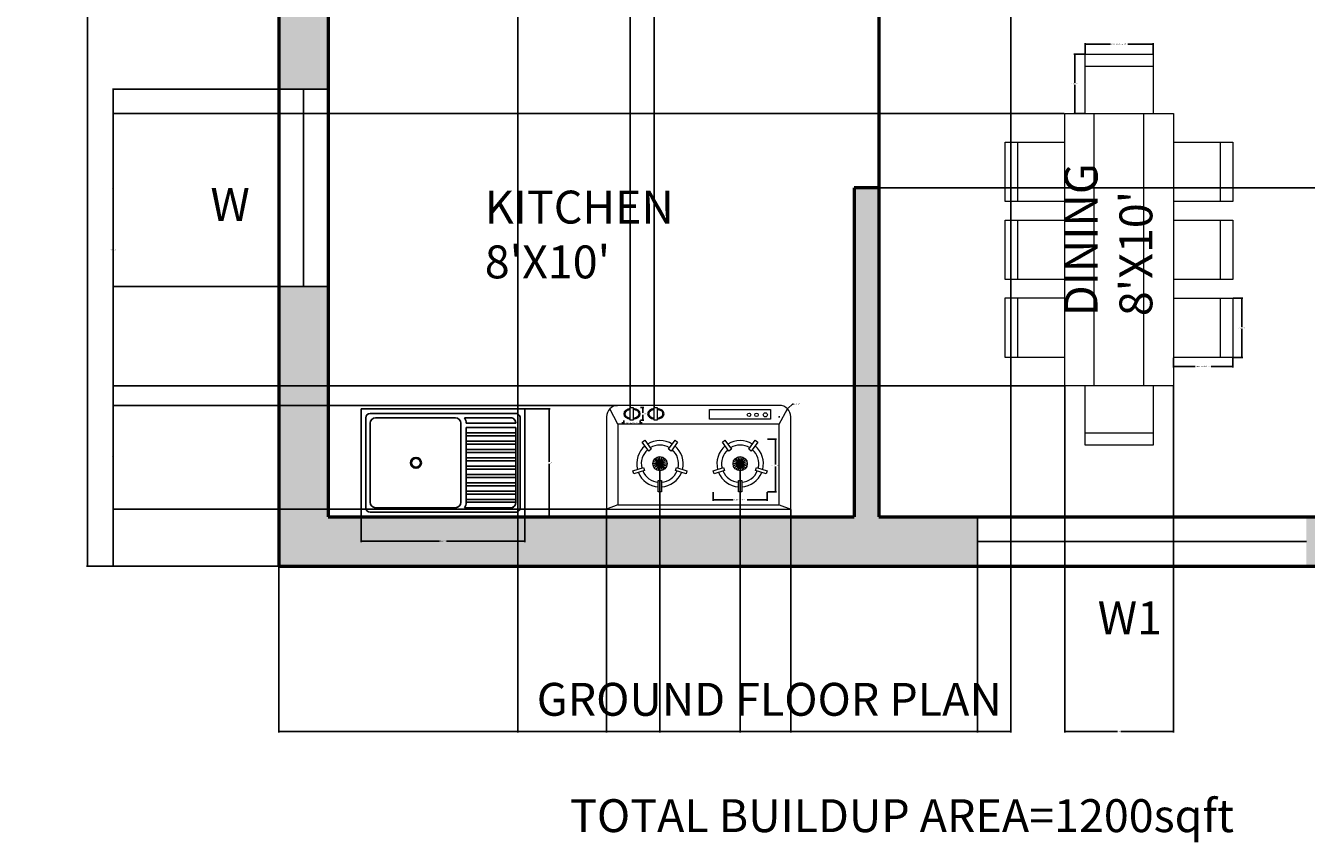
# Model space of a CAD drawing. Units: inches. Extents: x -15 to 420, y -514 to 86.
# Tile 1 of 8: x -15 to 218, y -514 to -365. Entities that reach past the tile are written whole.
import ezdxf

# ---------------------------------------------------------------- set-up
doc = ezdxf.new("R2010")
doc.units = ezdxf.units.IN
doc.header["$MEASUREMENT"] = 0
for name, color, linetype, lineweight in [('A-ANNO-DIMS', 2, 'Continuous', 18), ('A-ANNO-TEXT', 7, 'Continuous', 18), ('A-AREA-IDEN', 7, 'Continuous', 25), ('A-EQPM', 8, 'Continuous', 18), ('A-FLOR-FIXT', 9, 'Continuous', 25), ('A-FURN', 8, 'Continuous', 18), ('A-GLAZ', 41, 'Continuous', 25), ('A-WALL', 7, 'Continuous', 50), ('A-WALL-PATT', 8, 'Continuous', 13)]:
    doc.layers.add(name, color=color, linetype=linetype, lineweight=lineweight)
doc.styles.get("Standard").update_dxf_attribs({"font": 'arial.ttf'})
doc.dimstyles.get("Standard").update_dxf_attribs({"dimtxt": 0.18, "dimasz": 0.18, "dimexe": 0.18, "dimexo": 0.0625, "dimgap": 0.09, "dimtad": 0, "dimtih": 1, "dimtoh": 1, "dimdec": 0, "dimzin": 0, "dimdsep": 46, "dimlunit": 3, "dimtxsty": 'Standard', "dimcen": 0.09, "dimadec": 0, "dimazin": 0, "dimtfac": 1, "dimtdec": 0, "dimtofl": 0, "dimtmove": 0, "dimatfit": 3, "dimfxl": 1, "dimtolj": 1, "dimtzin": 0, "dimarcsym": 0})

# ---------------------------------------------------------------- blocks, each defined once
blk = doc.blocks.new('*D2')
at = {"layer": 'A-ANNO-DIMS', "color": 0, "lineweight": -2, "transparency": 16777216}
for p, q in [((30.86, 13.12), (-4.15, 13.12)), ((-3.97, 12.94), (-3.97, -222.22)), ((-3.97, -463.7), (-3.97, -228.53)), ((30.86, -463.88), (-4.15, -463.88))]:
    blk.add_line(p, q, dxfattribs=at)
at = {"layer": 'A-ANNO-DIMS', "color": 0, "transparency": 16777216}
for points in [[(-4, 12.94), (-3.94, 12.94), (-3.97, 13.12)], [(-4, -463.7), (-3.94, -463.7), (-3.97, -463.88)]]:
    blk.add_solid(points, dxfattribs=at)
at = {"layer": 'Defpoints', "color": 0, "transparency": 16777216}
for p in [(30.92, 13.12), (-3.97, -463.88), (30.92, -463.88)]:
    blk.add_point(p, dxfattribs=at)
at = {"layer": 'A-ANNO-DIMS', "color": 0, "transparency": 16777216, "insert": (-3.97, -225.38), "char_height": 6, "attachment_point": 5}
blk.add_mtext('\\A1;39\'-9"', dxfattribs=at)
blk = doc.blocks.new('М12 540х820')
for p, q in [((0, 540), (-820, 540)), ((-820, 540), (-820, 0)), ((-45, 517.5), (-775, 517.5)), ((0, 0), (0, 540)), ((-797.5, 495), (-797.5, 45)), ((-775, 468), (-775, 72)), ((-347.5, 495), (-748, 495)), ((-320.5, 468), (-320.5, 72)), ((-301.7, 495), (-64.8, 495)), ((-293.7, 468), (-293.7, 472.5)), ((-293.7, 468), (-45, 468)), ((-45, 469.5), (-45, 468)), ((-22.5, 45), (-22.5, 495)), ((-293.7, 446.6), (-45, 446.6)), ((-293.7, 419.6), (-293.7, 446.6)), ((-293.7, 419.6), (-45, 419.6)), ((-293.7, 405), (-45, 405)), ((-293.7, 378), (-293.7, 405)), ((-45, 419.6), (-45, 446.6)), ((-45, 378), (-45, 405)), ((-293.7, 378), (-45, 378)), ((-293.7, 336.4), (-293.7, 363.4)), ((-293.7, 363.4), (-45, 363.4)), ((-293.7, 336.4), (-45, 336.4)), ((-293.7, 294.7), (-293.7, 321.7)), ((-293.7, 321.7), (-45, 321.7)), ((-45, 336.4), (-45, 363.4)), ((-45, 294.7), (-45, 321.7)), ((-293.7, 294.7), (-45, 294.7)), ((-293.7, 253.1), (-293.7, 280.1)), ((-293.7, 280.1), (-45, 280.1)), ((-45, 253.1), (-45, 280.1)), ((-293.7, 253.1), (-45, 253.1)), ((-293.7, 211.5), (-293.7, 238.5)), ((-293.7, 238.5), (-45, 238.5)), ((-293.7, 211.5), (-45, 211.5)), ((-293.7, 169.9), (-293.7, 196.9)), ((-293.7, 196.9), (-45, 196.9)), ((-45, 211.5), (-45, 238.5)), ((-45, 169.9), (-45, 196.9)), ((-293.7, 169.9), (-45, 169.9)), ((-293.7, 128.2), (-293.7, 155.2)), ((-293.7, 155.2), (-45, 155.2)), ((-45, 128.2), (-45, 155.2)), ((-293.7, 128.2), (-45, 128.2)), ((-293.7, 113.6), (-45, 113.6)), ((-293.7, 86.6), (-293.7, 113.6)), ((-293.7, 86.6), (-45, 86.6)), ((-293.7, 72), (-45, 72)), ((-45, 86.6), (-45, 113.6)), ((-45, 70.5), (-45, 72)), ((-820, 0), (0, 0)), ((-775, 22.5), (-45, 22.5)), ((-748, 45), (-347.5, 45)), ((-301.7, 45), (-64.8, 45))]:
    blk.add_line(p, q)
at = {"ltscale": 0.06}
for p, q in [((-820, 0), (-820, 540)), ((-820, 540), (0, 540)), ((0, 540), (0, 536.9)), ((0, 536.9), (0, 0)), ((-293.7, 446.6), (-45, 446.6)), ((-293.7, 405), (-293.7, 446.6)), ((-293.7, 363.4), (-293.7, 405)), ((-45, 446.6), (-45, 419.6)), ((-45, 419.6), (-45, 378)), ((-293.7, 321.7), (-293.7, 363.4)), ((-293.7, 280.1), (-293.7, 321.7)), ((-45, 378), (-45, 336.4)), ((-45, 336.4), (-45, 294.7)), ((-293.7, 238.5), (-293.7, 280.1)), ((-45, 294.7), (-45, 253.1)), ((-293.7, 196.9), (-293.7, 238.5)), ((-293.7, 155.2), (-293.7, 196.9)), ((-45, 253.1), (-45, 211.5)), ((-45, 211.5), (-45, 169.9)), ((-293.7, 113.6), (-293.7, 155.2)), ((-45, 169.9), (-45, 128.2)), ((-293.7, 72), (-293.7, 113.6)), ((-45, 72), (-293.7, 72)), ((-45, 128.2), (-45, 86.6)), ((-45, 86.6), (-45, 72)), ((0, 0), (-820, 0))]:
    blk.add_line(p, q, dxfattribs=at)
at = {"extrusion": (0, 0, -1)}
for centre, major_axis, start_param, end_param in [((-775, 495), (-15.9, 15.9), -0.785398, 0.785398), ((-775, 495), (-15.9, 15.9), -0.785398, 0.785398), ((-45, 495), (-15.9, -15.9), 2.356194, 3.926991), ((-45, 495), (-15.9, -15.9), 2.356194, 3.926991), ((-748, 468), (-19.1, -19.1), 0.785398, 2.356194), ((-748, 468), (-19.1, -19.1), 0.785398, 2.356194), ((-347.5, 468), (-19.1, 19.1), 0.785398, 2.356194), ((-347.5, 468), (-19.1, 19.1), 0.785398, 2.356194), ((-343.2, 468), (-35, 35), 1.779263, 2.356194), ((-343.2, 468), (-35, 35), 1.779263, 2.356192), ((-343.2, 468), (-35, 35), 2.356192, 2.356194), ((-72.3, 468.8), (-19.3, 19.3), 1.0328, 2.38382), ((-72.3, 468.8), (-19.3, 19.3), 1.0328, 1.064673), ((-72.3, 468.8), (-19.3, 19.3), 1.064673, 2.328569), ((-72.3, 468.8), (-19.3, 19.3), 2.328569, 2.38382), ((-545.5, 270), (-19.1, -19.1), 3.926991, 10.210176), ((-545.5, 270), (-19.1, -19.1), 3.926991, 10.210176), ((-545.5, 270), (-15.9, -15.9), 3.926991, 10.210176), ((-545.5, 270), (-15.9, -15.9), 3.926991, 10.210176), ((-748, 72), (-19.1, 19.1), 3.926991, 5.497787), ((-748, 72), (-19.1, 19.1), 3.926991, 5.497787), ((-347.5, 72), (-19.1, -19.1), 3.926991, 5.497787), ((-347.5, 72), (-19.1, -19.1), 3.926991, 5.497787), ((-343.2, 72), (-35, -35), 3.926991, 4.503922), ((-343.2, 72), (-35, -35), 3.926991, 4.503922), ((-72.3, 71.2), (-19.3, -19.3), 3.899365, 5.250385), ((-72.3, 71.2), (-19.3, -19.3), 3.954617, 5.218512), ((-72.3, 71.2), (-19.3, -19.3), 3.899365, 3.954617), ((-775, 45), (-15.9, -15.9), 5.497787, 7.068583), ((-775, 45), (-15.9, -15.9), 5.497787, 7.068583), ((-72.3, 71.2), (-19.3, -19.3), 5.218512, 5.250385), ((-45, 45), (-15.9, 15.9), 2.356194, 3.926991), ((-45, 45), (-15.9, 15.9), 2.356194, 3.926991)]:
    blk.add_ellipse(centre, major_axis=major_axis, ratio=1, start_param=start_param, end_param=end_param, dxfattribs=at)
blk = doc.blocks.new('WIN-W1-60IN')
for p, q in [((0, 60), (0, 0)), ((4.5, 60), (4.5, 0)), ((9, 0), (9, 60))]:
    blk.add_line(p, q)
blk = doc.blocks.new('DINING-CHAIR-SIDE')
for p, q in [((0, 10.84), (10.83, 10.84)), ((0, 0), (0, 10.84)), ((2.26, 10.84), (2.26, 0)), ((10.83, 0), (0, 0))]:
    blk.add_line(p, q)
blk = doc.blocks.new('DINING-CHAIR-END')
for p, q in [((0, 0), (0, 10.84)), ((12.42, 10.84), (12.42, 0)), ((0, 2.26), (12.42, 2.26)), ((12.42, 0), (0, 0))]:
    blk.add_line(p, q)
blk = doc.blocks.new('COOKTOP-BURNER')
for p, q in [((1.71, 9.07), (2.18, 9.4)), ((2.18, 9.4), (3.38, 7.75)), ((6.51, 7.75), (7.71, 9.4)), ((7.71, 9.4), (8.18, 9.07)), ((2.91, 7.42), (1.71, 9.07)), ((3.38, 7.75), (2.91, 7.42)), ((6.98, 7.42), (6.51, 7.75)), ((8.18, 9.07), (6.98, 7.42)), ((4.95, 5.11), (3.65, 5.11)), ((4.95, 5.11), (3.71, 5.51)), ((4.95, 5.11), (3.71, 4.71)), ((4.95, 5.11), (3.9, 5.87)), ((4.95, 5.11), (3.9, 4.34)), ((4.95, 5.11), (4.18, 6.15)), ((4.95, 5.11), (4.18, 4.06)), ((4.95, 5.11), (4.54, 6.34)), ((4.95, 5.11), (4.54, 3.87)), ((4.95, 5.11), (4.95, 6.4)), ((4.95, 5.11), (5.35, 6.34)), ((4.95, 5.11), (5.71, 6.15)), ((4.95, 5.11), (5.99, 5.87)), ((4.95, 5.11), (6.18, 5.51)), ((4.95, 5.11), (6.24, 5.11)), ((4.95, 5.11), (6.18, 4.71)), ((4.95, 5.11), (5.99, 4.34)), ((4.95, 5.11), (5.71, 4.06)), ((4.95, 5.11), (5.35, 3.87)), ((4.95, 5.11), (4.95, 3.81)), ((0, 3.8), (1.94, 4.43)), ((0.18, 3.25), (0, 3.8)), ((2.12, 3.89), (0.18, 3.25)), ((1.94, 4.43), (2.12, 3.89)), ((7.77, 3.89), (7.95, 4.43)), ((9.71, 3.25), (7.77, 3.89)), ((7.95, 4.43), (9.89, 3.8)), ((9.89, 3.8), (9.71, 3.25)), ((4.66, 2.04), (5.23, 2.04)), ((4.66, 0), (4.66, 2.04)), ((5.23, 2.04), (5.23, 0)), ((5.23, 0), (4.66, 0))]:
    blk.add_line(p, q)
blk.add_circle((4.95, 5.11), 1.3)
for radius, start, end in [(4.24, 57.8765, 122.1235), (4.24, 129.8765, 194.1235), (3.4, 130.8365, 193.1635), (3.4, 58.8365, 121.1635), (3.4, 346.8365, 49.1635), (4.24, 345.8765, 50.1235), (4.24, 201.8765, 266.1235), (3.4, 202.8365, 265.1635), (3.4, 274.8365, 337.1635), (4.24, 273.8765, 338.1235)]:
    blk.add_arc((4.95, 5.11), radius, start, end)
blk = doc.blocks.new('COOKTOP-CONTROL')
for p, q in [((1.2, 0), (1.2, 2.33)), ((1.2, 2.33), (1.74, 2.33)), ((1.74, 2.33), (1.74, 0)), ((1.74, 0), (1.2, 0))]:
    blk.add_line(p, q)
for major_axis, start_param, end_param in [((1.5, 0), 1.774361, 4.508825), ((-1.5, 0), 1.73081, 4.552375)]:
    blk.add_ellipse((1.5, 1.17), major_axis=major_axis, ratio=0.671641, start_param=start_param, end_param=end_param)
for points, knots in [([(1.2, 1.95), (1.13, 1.94), (1.06, 1.92), (0.9, 1.88), (0.81, 1.85), (0.65, 1.78), (0.58, 1.73), (0.46, 1.64), (0.4, 1.59), (0.32, 1.49), (0.28, 1.44), (0.24, 1.34), (0.22, 1.29), (0.21, 1.18), (0.21, 1.13), (0.23, 1.03), (0.25, 0.98), (0.3, 0.88), (0.34, 0.83), (0.43, 0.73), (0.49, 0.68), (0.62, 0.59), (0.7, 0.55), (0.86, 0.48), (0.94, 0.45), (1.09, 0.42), (1.14, 0.4), (1.2, 0.4)], [8.079302, 8.079302, 8.079302, 8.079302, 8.245651, 8.245651, 8.463703, 8.463703, 8.681755, 8.681755, 8.899807, 8.899807, 9.117859, 9.117859, 9.33591, 9.33591, 9.553962, 9.553962, 9.772014, 9.772014, 9.990066, 9.990066, 10.208118, 10.208118, 10.426169, 10.426169, 10.644221, 10.644221, 10.770253, 10.770253, 10.770253, 10.770253]), ([(1.74, 0.39), (1.8, 0.39), (1.86, 0.4), (2, 0.43), (2.09, 0.46), (2.26, 0.53), (2.34, 0.56), (2.48, 0.65), (2.54, 0.69), (2.64, 0.79), (2.68, 0.84), (2.75, 0.95), (2.77, 1), (2.79, 1.09), (2.8, 1.13), (2.8, 1.17), (2.8, 1.22), (2.79, 1.28), (2.76, 1.38), (2.73, 1.43), (2.66, 1.53), (2.61, 1.58), (2.51, 1.68), (2.44, 1.72), (2.3, 1.81), (2.22, 1.84), (2.04, 1.9), (1.95, 1.93), (1.82, 1.95), (1.78, 1.96), (1.74, 1.96)], [4.889299, 4.889299, 4.889299, 4.889299, 5.015191, 5.015191, 5.233243, 5.233243, 5.451295, 5.451295, 5.669347, 5.669347, 5.887399, 5.887399, 6.10545, 6.10545, 6.283185, 6.283185, 6.283185, 6.501237, 6.501237, 6.719289, 6.719289, 6.937341, 6.937341, 7.155392, 7.155392, 7.373444, 7.373444, 7.591496, 7.591496, 7.677072, 7.677072, 7.677072, 7.677072])]:
    blk.add_open_spline(points, degree=3, knots=knots)
blk = doc.blocks.new('*D31')
at = {"layer": 'A-ANNO-DIMS', "color": 0, "lineweight": -2, "transparency": 16777216}
for p, q in [((194.18, -425.9), (194.18, -427.64)), ((194.36, -427.46), (198.14, -427.46)), ((204.84, -427.46), (201.06, -427.46)), ((205.02, -425.9), (205.02, -427.64))]:
    blk.add_line(p, q, dxfattribs=at)
at = {"layer": 'A-ANNO-DIMS', "color": 0, "transparency": 16777216}
for points in [[(194.36, -427.43), (194.36, -427.49), (194.18, -427.46)], [(204.84, -427.43), (204.84, -427.49), (205.02, -427.46)]]:
    blk.add_solid(points, dxfattribs=at)
at = {"layer": 'Defpoints', "color": 0, "transparency": 16777216}
for p in [(194.18, -425.83), (194.18, -427.46), (205.02, -425.83)]:
    blk.add_point(p, dxfattribs=at)
at = {"layer": 'A-ANNO-DIMS', "color": 0, "transparency": 16777216, "insert": (199.6, -427.46), "char_height": 0.18, "attachment_point": 5}
blk.add_mtext('\\A1;SIDE CHAIR 0\'-11" TYP.', dxfattribs=at)
blk = doc.blocks.new('*D32')
at = {"layer": 'A-ANNO-DIMS', "color": 0, "lineweight": -2, "transparency": 16777216}
for p, q in [((205.08, -415), (206.82, -415)), ((206.64, -415.18), (206.64, -420.23)), ((206.64, -425.65), (206.64, -420.6)), ((205.08, -425.83), (206.82, -425.83))]:
    blk.add_line(p, q, dxfattribs=at)
at = {"layer": 'A-ANNO-DIMS', "color": 0, "transparency": 16777216}
for points in [[(206.61, -415.18), (206.67, -415.18), (206.64, -415)], [(206.61, -425.65), (206.67, -425.65), (206.64, -425.83)]]:
    blk.add_solid(points, dxfattribs=at)
at = {"layer": 'Defpoints', "color": 0, "transparency": 16777216}
for p in [(205.02, -415), (205.02, -425.83), (206.64, -425.83)]:
    blk.add_point(p, dxfattribs=at)
at = {"layer": 'A-ANNO-DIMS', "color": 0, "transparency": 16777216, "insert": (206.64, -420.42), "char_height": 0.18, "attachment_point": 5}
blk.add_mtext('\\A1;0\'-11" TYP.', dxfattribs=at)
blk = doc.blocks.new('*D33')
at = {"layer": 'A-ANNO-DIMS', "color": 0, "lineweight": -2, "transparency": 16777216}
for p, q in [((178.04, -370.47), (178.04, -368.49)), ((178.22, -368.67), (182.68, -368.67)), ((190.28, -368.67), (185.82, -368.67)), ((190.46, -370.47), (190.46, -368.49))]:
    blk.add_line(p, q, dxfattribs=at)
at = {"layer": 'A-ANNO-DIMS', "color": 0, "transparency": 16777216}
for points in [[(178.22, -368.64), (178.22, -368.7), (178.04, -368.67)], [(190.28, -368.64), (190.28, -368.7), (190.46, -368.67)]]:
    blk.add_solid(points, dxfattribs=at)
at = {"layer": 'Defpoints', "color": 0, "transparency": 16777216}
for p in [(178.04, -368.67), (178.04, -370.53), (190.46, -370.53)]:
    blk.add_point(p, dxfattribs=at)
at = {"layer": 'A-ANNO-DIMS', "color": 0, "transparency": 16777216, "insert": (184.25, -368.67), "char_height": 0.18, "attachment_point": 5}
blk.add_mtext('\\A1;END CHAIR 1\'-0 1/2" TYP.', dxfattribs=at)
blk = doc.blocks.new('*D34')
at = {"layer": 'A-ANNO-DIMS', "color": 0, "lineweight": -2, "transparency": 16777216}
for p, q in [((177.98, -370.53), (176, -370.53)), ((176.18, -370.71), (176.18, -375.76)), ((176.18, -381.18), (176.18, -376.13)), ((177.98, -381.36), (176, -381.36))]:
    blk.add_line(p, q, dxfattribs=at)
at = {"layer": 'A-ANNO-DIMS', "color": 0, "transparency": 16777216}
for points in [[(176.15, -370.71), (176.21, -370.71), (176.18, -370.53)], [(176.15, -381.18), (176.21, -381.18), (176.18, -381.36)]]:
    blk.add_solid(points, dxfattribs=at)
at = {"layer": 'Defpoints', "color": 0, "transparency": 16777216}
for p in [(178.04, -370.53), (176.18, -381.36), (178.04, -381.36)]:
    blk.add_point(p, dxfattribs=at)
at = {"layer": 'A-ANNO-DIMS', "color": 0, "transparency": 16777216, "insert": (176.18, -375.95), "char_height": 0.18, "attachment_point": 5}
blk.add_mtext('\\A1;0\'-11" TYP.', dxfattribs=at)
blk = doc.blocks.new('*D39')
at = {"layer": 'A-ANNO-DIMS', "color": 0, "lineweight": -2, "transparency": 16777216}
for p, q in [((110.15, -450.39), (110.15, -451.99)), ((120.04, -450.39), (120.04, -451.99)), ((110.33, -451.81), (113.83, -451.81)), ((119.86, -451.81), (116.37, -451.81))]:
    blk.add_line(p, q, dxfattribs=at)
at = {"layer": 'A-ANNO-DIMS', "color": 0, "transparency": 16777216}
for points in [[(110.33, -451.78), (110.33, -451.84), (110.15, -451.81)], [(119.86, -451.78), (119.86, -451.84), (120.04, -451.81)]]:
    blk.add_solid(points, dxfattribs=at)
at = {"layer": 'Defpoints', "color": 0, "transparency": 16777216}
for p in [(110.15, -450.33), (120.04, -450.33), (120.04, -451.81)]:
    blk.add_point(p, dxfattribs=at)
at = {"layer": 'A-ANNO-DIMS', "color": 0, "transparency": 16777216, "insert": (115.1, -451.81), "char_height": 0.18, "attachment_point": 5}
blk.add_mtext('\\A1;BURNER 0\'-10" TYP.', dxfattribs=at)
blk = doc.blocks.new('*D40')
at = {"layer": 'A-ANNO-DIMS', "color": 0, "lineweight": -2, "transparency": 16777216}
for p, q in [((120.11, -440.76), (121.71, -440.76)), ((121.53, -440.94), (121.53, -445.36)), ((121.53, -450.15), (121.53, -445.73)), ((120.11, -450.33), (121.71, -450.33))]:
    blk.add_line(p, q, dxfattribs=at)
at = {"layer": 'A-ANNO-DIMS', "color": 0, "transparency": 16777216}
for points in [[(121.5, -440.94), (121.56, -440.94), (121.53, -440.76)], [(121.5, -450.15), (121.56, -450.15), (121.53, -450.33)]]:
    blk.add_solid(points, dxfattribs=at)
at = {"layer": 'Defpoints', "color": 0, "transparency": 16777216}
for p in [(120.04, -440.76), (121.53, -440.76), (120.04, -450.33)]:
    blk.add_point(p, dxfattribs=at)
at = {"layer": 'A-ANNO-DIMS', "color": 0, "transparency": 16777216, "insert": (121.53, -445.54), "char_height": 0.18, "attachment_point": 5}
blk.add_mtext('\\A1;0\'-9 1/2" TYP.', dxfattribs=at)
blk = doc.blocks.new('*D41')
at = {"layer": 'A-ANNO-DIMS', "color": 0, "lineweight": -2, "transparency": 16777216}
for p, q in [((93.68, -437.74), (93.5, -437.74)), ((93.86, -437.35), (93.86, -437.92)), ((96.87, -437.35), (96.87, -437.92)), ((97.05, -437.74), (97.23, -437.74))]:
    blk.add_line(p, q, dxfattribs=at)
at = {"layer": 'A-ANNO-DIMS', "color": 0, "transparency": 16777216}
for points in [[(93.68, -437.71), (93.68, -437.77), (93.86, -437.74)], [(97.05, -437.71), (97.05, -437.77), (96.87, -437.74)]]:
    blk.add_solid(points, dxfattribs=at)
at = {"layer": 'Defpoints', "color": 0, "transparency": 16777216}
for p in [(93.86, -437.29), (96.87, -437.29), (96.87, -437.74)]:
    blk.add_point(p, dxfattribs=at)
at = {"layer": 'A-ANNO-DIMS', "color": 0, "transparency": 16777216, "insert": (95.37, -437.74), "char_height": 0.18, "attachment_point": 5}
blk.add_mtext('\\A1;CONTROL 0\'-3" TYP.', dxfattribs=at)
blk = doc.blocks.new('*D42')
at = {"layer": 'A-ANNO-DIMS', "color": 0, "lineweight": -2, "transparency": 16777216}
for p, q in [((96.94, -434.96), (97.5, -434.96)), ((97.32, -435.14), (97.32, -435.94)), ((97.32, -437.11), (97.32, -436.31)), ((96.94, -437.29), (97.5, -437.29))]:
    blk.add_line(p, q, dxfattribs=at)
at = {"layer": 'A-ANNO-DIMS', "color": 0, "transparency": 16777216}
for points in [[(97.29, -435.14), (97.35, -435.14), (97.32, -434.96)], [(97.29, -437.11), (97.35, -437.11), (97.32, -437.29)]]:
    blk.add_solid(points, dxfattribs=at)
at = {"layer": 'Defpoints', "color": 0, "transparency": 16777216}
for p in [(96.87, -434.96), (97.32, -434.96), (96.87, -437.29)]:
    blk.add_point(p, dxfattribs=at)
at = {"layer": 'A-ANNO-DIMS', "color": 0, "transparency": 16777216, "insert": (97.32, -436.12), "char_height": 0.18, "attachment_point": 5}
blk.add_mtext('\\A1;0\'-2 1/2" TYP.', dxfattribs=at)
blk = doc.blocks.new('*D43')
at = {"layer": 'A-ANNO-DIMS', "color": 0, "lineweight": -2, "transparency": 16777216}
for p, q in [((45.95, -454.94), (45.95, -459.54)), ((75.8, -454.94), (75.8, -459.54)), ((46.13, -459.36), (60.22, -459.36)), ((75.62, -459.36), (61.54, -459.36))]:
    blk.add_line(p, q, dxfattribs=at)
at = {"layer": 'A-ANNO-DIMS', "color": 0, "transparency": 16777216}
for points in [[(46.13, -459.33), (46.13, -459.39), (45.95, -459.36)], [(75.62, -459.33), (75.62, -459.39), (75.8, -459.36)]]:
    blk.add_solid(points, dxfattribs=at)
at = {"layer": 'Defpoints', "color": 0, "transparency": 16777216}
for p in [(45.95, -454.88), (75.8, -454.88), (75.8, -459.36)]:
    blk.add_point(p, dxfattribs=at)
at = {"layer": 'A-ANNO-DIMS', "color": 0, "transparency": 16777216, "insert": (60.88, -459.36), "char_height": 0.18, "attachment_point": 5}
blk.add_mtext('\\A1;SINK 2\'-6"', dxfattribs=at)
blk = doc.blocks.new('*D44')
at = {"layer": 'A-ANNO-DIMS', "color": 0, "lineweight": -2, "transparency": 16777216}
for p, q in [((75.87, -435.22), (80.46, -435.22)), ((80.28, -435.4), (80.28, -444.87)), ((80.28, -454.7), (80.28, -445.23)), ((75.87, -454.88), (80.46, -454.88))]:
    blk.add_line(p, q, dxfattribs=at)
at = {"layer": 'A-ANNO-DIMS', "color": 0, "transparency": 16777216}
for points in [[(80.25, -435.4), (80.31, -435.4), (80.28, -435.22)], [(80.25, -454.7), (80.31, -454.7), (80.28, -454.88)]]:
    blk.add_solid(points, dxfattribs=at)
at = {"layer": 'Defpoints', "color": 0, "transparency": 16777216}
for p in [(75.8, -435.22), (80.28, -435.22), (75.8, -454.88)]:
    blk.add_point(p, dxfattribs=at)
at = {"layer": 'A-ANNO-DIMS', "color": 0, "transparency": 16777216, "insert": (80.28, -445.05), "char_height": 0.18, "attachment_point": 5}
blk.add_mtext('\\A1;1\'-7 1/2"', dxfattribs=at)
blk = doc.blocks.new('*D45')
at = {"layer": 'A-ANNO-DIMS', "color": 0, "lineweight": -2, "transparency": 16777216}
for p, q in [((30.86, -376.88), (0.54, -376.88)), ((0.72, -377.06), (0.72, -394.7)), ((0.72, -412.7), (0.72, -395.06)), ((30.86, -412.88), (0.54, -412.88))]:
    blk.add_line(p, q, dxfattribs=at)
at = {"layer": 'A-ANNO-DIMS', "color": 0, "transparency": 16777216}
for points in [[(0.69, -377.06), (0.75, -377.06), (0.72, -376.88)], [(0.69, -412.7), (0.75, -412.7), (0.72, -412.88)]]:
    blk.add_solid(points, dxfattribs=at)
at = {"layer": 'Defpoints', "color": 0, "transparency": 16777216}
for p in [(30.92, -376.88), (0.72, -412.88), (30.92, -412.88)]:
    blk.add_point(p, dxfattribs=at)
at = {"layer": 'A-ANNO-DIMS', "color": 0, "transparency": 16777216, "insert": (0.72, -394.88), "char_height": 0.18, "attachment_point": 5}
blk.add_mtext('\\A1;3\'-0"', dxfattribs=at)
blk = doc.blocks.new('*D49')
at = {"layer": 'A-ANNO-DIMS', "color": 0, "lineweight": -2, "transparency": 16777216}
for p, q in [((74.51, -330.44), (74.51, -494.26)), ((164.51, -330.44), (164.51, -494.26)), ((74.69, -494.08), (119.18, -494.08)), ((164.33, -494.08), (119.84, -494.08))]:
    blk.add_line(p, q, dxfattribs=at)
at = {"layer": 'A-ANNO-DIMS', "color": 0, "transparency": 16777216}
for points in [[(74.69, -494.05), (74.69, -494.11), (74.51, -494.08)], [(164.33, -494.05), (164.33, -494.11), (164.51, -494.08)]]:
    blk.add_solid(points, dxfattribs=at)
at = {"layer": 'Defpoints', "color": 0, "transparency": 16777216}
for p in [(74.51, -330.38), (164.51, -330.38), (164.51, -494.08)]:
    blk.add_point(p, dxfattribs=at)
at = {"layer": 'A-ANNO-DIMS', "color": 0, "transparency": 16777216, "insert": (119.51, -494.08), "char_height": 0.18, "attachment_point": 5}
blk.add_mtext('\\A1;7\'-6"', dxfattribs=at)
blk = doc.blocks.new('*D52')
at = {"layer": 'A-ANNO-DIMS', "color": 0, "lineweight": -2, "transparency": 16777216}
for p, q in [((140.49, -357.15), (419.8, -357.15)), ((419.62, -357.33), (419.62, -375.83)), ((419.62, -394.7), (419.62, -376.2)), ((140.49, -394.88), (419.8, -394.88))]:
    blk.add_line(p, q, dxfattribs=at)
at = {"layer": 'A-ANNO-DIMS', "color": 0, "transparency": 16777216}
for points in [[(419.59, -357.33), (419.65, -357.33), (419.62, -357.15)], [(419.59, -394.7), (419.65, -394.7), (419.62, -394.88)]]:
    blk.add_solid(points, dxfattribs=at)
at = {"layer": 'Defpoints', "color": 0, "transparency": 16777216}
for p in [(140.42, -357.15), (140.42, -394.88), (419.62, -394.88)]:
    blk.add_point(p, dxfattribs=at)
at = {"layer": 'A-ANNO-DIMS', "color": 0, "transparency": 16777216, "insert": (419.62, -376.01), "char_height": 0.18, "attachment_point": 5}
blk.add_mtext('\\A1;3\'-1 1/2"', dxfattribs=at)
blk = doc.blocks.new('*D53')
at = {"layer": 'A-ANNO-DIMS', "color": 0, "lineweight": -2, "transparency": 16777216}
for p, q in [((174.32, -431.09), (174.32, -494.26)), ((194.18, -431.09), (194.18, -494.26)), ((174.5, -494.08), (183.93, -494.08)), ((194, -494.08), (184.57, -494.08))]:
    blk.add_line(p, q, dxfattribs=at)
at = {"layer": 'A-ANNO-DIMS', "color": 0, "transparency": 16777216}
for points in [[(174.5, -494.05), (174.5, -494.11), (174.32, -494.08)], [(194, -494.05), (194, -494.11), (194.18, -494.08)]]:
    blk.add_solid(points, dxfattribs=at)
at = {"layer": 'Defpoints', "color": 0, "transparency": 16777216}
for p in [(174.32, -431.02), (194.18, -431.02), (194.18, -494.08)]:
    blk.add_point(p, dxfattribs=at)
at = {"layer": 'A-ANNO-DIMS', "color": 0, "transparency": 16777216, "insert": (184.25, -494.08), "char_height": 0.18, "attachment_point": 5}
blk.add_mtext('\\A1;1\'-8"', dxfattribs=at)
blk = doc.blocks.new('*D54')
at = {"layer": 'A-ANNO-DIMS', "color": 0, "lineweight": -2, "transparency": 16777216}
for p, q in [((174.25, -381.36), (0.54, -381.36)), ((0.72, -381.54), (0.72, -406.01)), ((0.72, -430.84), (0.72, -406.38)), ((174.25, -431.02), (0.54, -431.02))]:
    blk.add_line(p, q, dxfattribs=at)
at = {"layer": 'A-ANNO-DIMS', "color": 0, "transparency": 16777216}
for points in [[(0.69, -381.54), (0.75, -381.54), (0.72, -381.36)], [(0.69, -430.84), (0.75, -430.84), (0.72, -431.02)]]:
    blk.add_solid(points, dxfattribs=at)
at = {"layer": 'Defpoints', "color": 0, "transparency": 16777216}
for p in [(0.72, -381.36), (174.32, -381.36), (174.32, -431.02)]:
    blk.add_point(p, dxfattribs=at)
at = {"layer": 'A-ANNO-DIMS', "color": 0, "transparency": 16777216, "insert": (0.72, -406.19), "char_height": 0.18, "attachment_point": 5}
blk.add_mtext('\\A1;4\'-1 1/2"', dxfattribs=at)
blk = doc.blocks.new('*D55')
at = {"layer": 'A-ANNO-DIMS', "color": 0, "lineweight": -2, "transparency": 16777216}
for p, q in [((90.71, -453.56), (90.71, -494.26)), ((124.34, -453.56), (124.34, -494.26)), ((90.89, -494.08), (106.99, -494.08)), ((124.16, -494.08), (108.07, -494.08))]:
    blk.add_line(p, q, dxfattribs=at)
at = {"layer": 'A-ANNO-DIMS', "color": 0, "transparency": 16777216}
for points in [[(90.89, -494.05), (90.89, -494.11), (90.71, -494.08)], [(124.16, -494.05), (124.16, -494.11), (124.34, -494.08)]]:
    blk.add_solid(points, dxfattribs=at)
at = {"layer": 'Defpoints', "color": 0, "transparency": 16777216}
for p in [(90.71, -453.5), (124.34, -453.5), (124.34, -494.08)]:
    blk.add_point(p, dxfattribs=at)
at = {"layer": 'A-ANNO-DIMS', "color": 0, "transparency": 16777216, "insert": (107.53, -494.08), "char_height": 0.18, "attachment_point": 5}
blk.add_mtext('\\A1;2\'-9 1/2"', dxfattribs=at)
blk = doc.blocks.new('*D56')
at = {"layer": 'A-ANNO-DIMS', "color": 0, "lineweight": -2, "transparency": 16777216}
for p, q in [((92.75, -434.58), (0.54, -434.58)), ((0.72, -434.76), (0.72, -443.86)), ((0.72, -453.32), (0.72, -444.22)), ((90.65, -453.5), (0.54, -453.5))]:
    blk.add_line(p, q, dxfattribs=at)
at = {"layer": 'A-ANNO-DIMS', "color": 0, "transparency": 16777216}
for points in [[(0.69, -434.76), (0.75, -434.76), (0.72, -434.58)], [(0.69, -453.32), (0.75, -453.32), (0.72, -453.5)]]:
    blk.add_solid(points, dxfattribs=at)
at = {"layer": 'Defpoints', "color": 0, "transparency": 16777216}
for p in [(92.81, -434.58), (0.72, -453.5), (90.71, -453.5)]:
    blk.add_point(p, dxfattribs=at)
at = {"layer": 'A-ANNO-DIMS', "color": 0, "transparency": 16777216, "insert": (0.72, -444.04), "char_height": 0.18, "attachment_point": 5}
blk.add_mtext('\\A1;1\'-7"', dxfattribs=at)
blk = doc.blocks.new('*D57')
at = {"layer": 'A-ANNO-DIMS', "color": 0, "lineweight": -2, "transparency": 16777216}
for p, q in [((100.46, -445.28), (100.46, -494.26)), ((115.1, -445.28), (115.1, -494.26)), ((100.64, -494.08), (107.25, -494.08)), ((114.92, -494.08), (108.31, -494.08))]:
    blk.add_line(p, q, dxfattribs=at)
at = {"layer": 'A-ANNO-DIMS', "color": 0, "transparency": 16777216}
for points in [[(100.64, -494.05), (100.64, -494.11), (100.46, -494.08)], [(114.92, -494.05), (114.92, -494.11), (115.1, -494.08)]]:
    blk.add_solid(points, dxfattribs=at)
at = {"layer": 'Defpoints', "color": 0, "transparency": 16777216}
for p in [(100.46, -445.22), (115.1, -445.22), (115.1, -494.08)]:
    blk.add_point(p, dxfattribs=at)
at = {"layer": 'A-ANNO-DIMS', "color": 0, "transparency": 16777216, "insert": (107.78, -494.08), "char_height": 0.18, "attachment_point": 5}
blk.add_mtext('\\A1;1\'-2 1/2"', dxfattribs=at)
blk = doc.blocks.new('*D58')
at = {"layer": 'A-ANNO-DIMS', "color": 0, "lineweight": -2, "transparency": 16777216}
for p, q in [((95.06, -434.9), (95.06, 43.5)), ((95.24, 43.32), (96.7, 43.32)), ((99.24, 43.32), (97.78, 43.32)), ((99.42, -434.9), (99.42, 43.5))]:
    blk.add_line(p, q, dxfattribs=at)
at = {"layer": 'A-ANNO-DIMS', "color": 0, "transparency": 16777216}
for points in [[(95.24, 43.35), (95.24, 43.29), (95.06, 43.32)], [(99.24, 43.35), (99.24, 43.29), (99.42, 43.32)]]:
    blk.add_solid(points, dxfattribs=at)
at = {"layer": 'Defpoints', "color": 0, "transparency": 16777216}
for p in [(99.42, 43.32), (95.06, -434.96), (99.42, -434.96)]:
    blk.add_point(p, dxfattribs=at)
at = {"layer": 'A-ANNO-DIMS', "color": 0, "transparency": 16777216, "insert": (97.24, 43.32), "char_height": 0.18, "attachment_point": 5}
blk.add_mtext('\\A1;0\'-4 1/2"', dxfattribs=at)
blk = doc.blocks.new('*D64')
at = {"layer": 'A-ANNO-DIMS', "color": 0, "lineweight": -2, "transparency": 16777216}
for p, q in [((30.86, -412.88), (0.54, -412.88)), ((0.72, -413.06), (0.72, -438.2)), ((0.72, -463.7), (0.72, -438.56)), ((30.86, -463.88), (0.54, -463.88))]:
    blk.add_line(p, q, dxfattribs=at)
at = {"layer": 'A-ANNO-DIMS', "color": 0, "transparency": 16777216}
for points in [[(0.69, -413.06), (0.75, -413.06), (0.72, -412.88)], [(0.69, -463.7), (0.75, -463.7), (0.72, -463.88)]]:
    blk.add_solid(points, dxfattribs=at)
at = {"layer": 'Defpoints', "color": 0, "transparency": 16777216}
for p in [(0.72, -412.88), (30.92, -412.88), (30.92, -463.88)]:
    blk.add_point(p, dxfattribs=at)
at = {"layer": 'A-ANNO-DIMS', "color": 0, "transparency": 16777216, "insert": (0.72, -438.38), "char_height": 0.18, "attachment_point": 5}
blk.add_mtext('\\A1;4\'-3"', dxfattribs=at)
blk = doc.blocks.new('*D65')
at = {"layer": 'A-ANNO-DIMS', "color": 0, "lineweight": -2, "transparency": 16777216}
for p, q in [((30.92, -463.94), (30.92, -494.26)), ((158.42, -463.94), (158.42, -494.26)), ((31.1, -494.08), (94.07, -494.08)), ((158.24, -494.08), (95.28, -494.08))]:
    blk.add_line(p, q, dxfattribs=at)
at = {"layer": 'A-ANNO-DIMS', "color": 0, "transparency": 16777216}
for points in [[(31.1, -494.05), (31.1, -494.11), (30.92, -494.08)], [(158.24, -494.05), (158.24, -494.11), (158.42, -494.08)]]:
    blk.add_solid(points, dxfattribs=at)
at = {"layer": 'Defpoints', "color": 0, "transparency": 16777216}
for p in [(30.92, -463.88), (158.42, -463.88), (158.42, -494.08)]:
    blk.add_point(p, dxfattribs=at)
at = {"layer": 'A-ANNO-DIMS', "color": 0, "transparency": 16777216, "insert": (94.67, -494.08), "char_height": 0.18, "attachment_point": 5}
blk.add_mtext('\\A1;10\'-7 1/2"', dxfattribs=at)
blk = doc.blocks.new('*D72')
at = {"layer": 'A-ANNO-DIMS', "color": 0, "lineweight": -2, "transparency": 16777216}
for p, q in [((124.65, -434.33), (123.87, -435.09)), ((124.83, -434.33), (124.65, -434.33)), ((122.15, -436.68), (122.33, -436.68)), ((122.24, -436.77), (122.24, -436.59))]:
    blk.add_line(p, q, dxfattribs=at)
at = {"layer": 'A-ANNO-DIMS', "color": 0, "transparency": 16777216}
blk.add_solid([(123.85, -435.07), (123.89, -435.11), (123.74, -435.21)], dxfattribs=at)
at = {"layer": 'Defpoints', "color": 0, "transparency": 16777216}
for p in [(122.24, -436.68), (123.74, -435.21)]:
    blk.add_point(p, dxfattribs=at)
at = {"layer": 'A-ANNO-DIMS', "color": 0, "transparency": 16777216, "insert": (125.44, -434.33), "char_height": 0.18, "attachment_point": 5}
blk.add_mtext('\\A1;2X R0\'-2"', dxfattribs=at)

msp = doc.modelspace()

# ---------------------------------------------------------------- hatches: boundary and pattern name
at = {"layer": 'A-WALL-PATT'}
h = msp.add_hatch(color=256, dxfattribs=at)
h.dxf.hatch_style = 1
h.paths.add_polyline_path([(266.67, -454.88), (240.92, -454.88), (240.92, -330.38), (236.42, -330.38), (236.42, -454.88), (218.42, -454.88), (218.42, -463.88), (266.67, -463.88)])
h.paths.add_polyline_path([(158.42, -454.88), (140.42, -454.88), (140.42, -394.88), (135.92, -394.88), (135.92, -454.88), (39.92, -454.88), (39.92, -412.88), (30.92, -412.88), (30.92, -463.88), (158.42, -463.88)])
h.paths.add_polyline_path([(39.92, -334.88), (135.92, -334.88), (135.92, -357.15), (140.42, -357.15), (140.42, -334.88), (173.95, -334.88), (173.95, -330.38), (39.92, -330.38), (39.92, -250.88), (155.51, -250.88), (155.51, -246.38), (140.42, -246.38), (140.42, -205.38), (138.17, -205.38), (135.92, -205.38), (135.92, -246.38), (39.92, -246.38), (39.92, -222.38), (30.92, -222.38), (30.92, -376.88), (39.92, -376.88)])
h.paths.add_polyline_path([(389.42, -382.88), (380.42, -382.88), (380.42, -454.88), (380.42, -463.88), (389.42, -463.88)])
h.paths.add_polyline_path([(352.42, -459.38), (352.42, -454.88), (326.67, -454.88), (326.67, -463.88), (352.42, -463.88)])
h.paths.add_polyline_path([(176.92, -169.88), (39.92, -169.88), (39.92, -112.88), (30.92, -112.88), (30.92, -198.38), (39.92, -198.38), (39.92, -174.38), (135.92, -174.38), (135.92, -177.38), (140.42, -177.38), (140.42, -174.38), (176.92, -174.38), (176.92, -172.13)])
h.paths.add_polyline_path([(39.92, 4.12), (93.92, 4.12), (93.92, 13.12), (30.92, 13.12), (30.92, -52.88), (39.92, -52.88)])
h.paths.add_polyline_path([(266.42, 13.12), (153.92, 13.12), (153.92, 4.12), (207.92, 4.12), (207.92, -169.88), (204.92, -169.88), (204.92, -174.38), (215.42, -174.38), (215.42, -169.88), (212.42, -169.88), (212.42, 4.12), (266.42, 4.12)])
h.paths.add_polyline_path([(389.42, 13.12), (326.42, 13.12), (326.42, 4.12), (380.42, 4.12), (380.42, -52.88), (389.42, -52.88)])
h.paths.add_polyline_path([(389.42, -112.88), (380.42, -112.88), (380.42, -169.88), (377.42, -169.88), (377.42, -174.38), (380.42, -174.38), (380.42, -198.38), (389.42, -198.38)])
h.paths.add_polyline_path([(349.42, -172.13), (349.42, -169.88), (243.42, -169.88), (243.42, -172.13), (243.42, -174.38), (279.92, -174.38), (279.92, -250.88), (380.42, -250.88), (380.42, -322.88), (389.42, -322.88), (389.42, -222.38), (380.42, -222.38), (380.42, -246.38), (284.42, -246.38), (284.42, -174.38), (349.42, -174.38)])

# ---------------------------------------------------------------- linework, layer by layer
at = {"layer": 'A-EQPM'}
for p, q in [((122.24, -434.58), (92.81, -434.58)), ((90.71, -436.68), (90.71, -453.5)), ((92.81, -437.99), (91.32, -435.2)), ((109.51, -435.31), (120.63, -435.31)), ((109.51, -437.11), (109.51, -435.31)), ((120.63, -435.31), (120.63, -437.11)), ((122.24, -437.99), (123.73, -435.2)), ((124.34, -453.5), (124.34, -436.68)), ((92.81, -437.99), (92.81, -452.7)), ((122.24, -437.99), (92.81, -437.99)), ((120.63, -437.11), (109.51, -437.11)), ((122.24, -452.7), (122.24, -437.99)), ((92.81, -452.7), (90.71, -453.5)), ((92.81, -452.7), (122.24, -452.7)), ((122.24, -452.7), (124.34, -453.5)), ((90.71, -453.5), (124.34, -453.5))]:
    msp.add_line(p, q, dxfattribs=at)
for centre, radius in [((116.72, -436.3), 0.311), ((118.09, -436.3), 0.311), ((119.7, -436.3), 0.373)]:
    msp.add_circle(centre, radius, dxfattribs=at)
for centre, start, end in [((92.81, -436.68), 90, 180), ((122.24, -436.68), 0, 90)]:
    msp.add_arc(centre, 2.1, start, end, dxfattribs=at)
at = {"layer": 'A-FURN'}
for p, q in [((174.32, -431.02), (174.32, -381.36)), ((174.32, -381.36), (194.18, -381.36)), ((179.73, -431.02), (179.73, -381.36)), ((188.76, -431.02), (188.76, -381.36)), ((194.18, -381.36), (194.18, -431.02)), ((194.18, -431.02), (174.32, -431.02))]:
    msp.add_line(p, q, dxfattribs=at)
at = {"layer": 'A-GLAZ'}
for p, q in [((30.92, -376.88), (30.92, -412.88)), ((39.92, -376.88), (30.92, -376.88)), ((35.42, -376.88), (35.42, -412.88)), ((39.92, -412.88), (39.92, -376.88)), ((30.92, -412.88), (39.92, -412.88)), ((158.42, -463.88), (158.42, -454.88))]:
    msp.add_line(p, q, dxfattribs=at)
at = {"layer": 'A-WALL'}
for p, q in [((30.92, 13.12), (30.92, -463.88)), ((39.92, -334.88), (39.92, -454.88)), ((140.42, -334.88), (140.42, -454.88)), ((140.42, -394.88), (135.92, -394.88)), ((135.92, -394.88), (135.92, -454.88)), ((39.92, -454.88), (135.92, -454.88)), ((140.42, -454.88), (236.42, -454.88)), ((30.92, -463.88), (389.42, -463.88))]:
    msp.add_line(p, q, dxfattribs=at)

# ---------------------------------------------------------------- block references
at = {"layer": 'A-EQPM'}
for name, p in [('COOKTOP-CONTROL', (93.86, -437.29)), ('COOKTOP-CONTROL', (98.22, -437.29)), ('COOKTOP-BURNER', (95.51, -450.33)), ('COOKTOP-BURNER', (110.15, -450.33))]:
    msp.add_blockref(name, p, dxfattribs=at)
at = {"layer": 'A-FLOR-FIXT', "xscale": 0.0364019794065407, "yscale": 0.0364019794065407, "zscale": 0.0364019794065407}
msp.add_blockref('М12 540х820', (75.8, -454.88), dxfattribs=at)
at = {"layer": 'A-FURN', "rotation": 180}
for name, p in [('DINING-CHAIR-END', (190.46, -370.53)), ('DINING-CHAIR-SIDE', (205.02, -386.55)), ('DINING-CHAIR-SIDE', (205.02, -400.78)), ('DINING-CHAIR-SIDE', (205.02, -415))]:
    msp.add_blockref(name, p, dxfattribs=at)
at = {"layer": 'A-FURN'}
for name, p in [('DINING-CHAIR-SIDE', (163.48, -397.39)), ('DINING-CHAIR-SIDE', (163.48, -411.61)), ('DINING-CHAIR-SIDE', (163.48, -425.83)), ('DINING-CHAIR-END', (178.04, -441.86))]:
    msp.add_blockref(name, p, dxfattribs=at)
at = {"layer": 'A-GLAZ', "rotation": 270}
msp.add_blockref('WIN-W1-60IN', (158.43, -454.88), dxfattribs=at)

# ---------------------------------------------------------------- texts
at = {"layer": 'A-ANNO-TEXT', "insert": (18.44, -394.92), "char_height": 6, "attachment_point": 1}
msp.add_mtext_dynamic_manual_height_columns('W', width=10.2557, gutter_width=1, heights=[0], dxfattribs=at)
at = {"layer": 'A-ANNO-TEXT', "char_height": 6, "attachment_point": 1}
for s, insert in [('W1', (180.35, -470.34)), ('GROUND FLOOR PLAN', (77.99, -485.19)), ('TOTAL BUILDUP AREA=1200sqft', (84.06, -506.41))]:
    msp.add_mtext(s, dxfattribs=dict(at, insert=insert))
at = {"layer": 'A-AREA-IDEN', "insert": (174.32, -418.31), "char_height": 6, "attachment_point": 1, "rotation": 90}
msp.add_mtext("DINING\\P8'X10'", dxfattribs=at)
at = {"layer": 'A-AREA-IDEN', "insert": (68.5, -395.41), "char_height": 6, "attachment_point": 1}
msp.add_mtext("KITCHEN\\P8'X10'", dxfattribs=at)

# ---------------------------------------------------------------- dimensions: what is measured, and where the dimension line sits
at = {"layer": 'A-ANNO-DIMS'}
for base, p1, p2, picture, middle in [((99.42, 43.32), (95.06, -434.96), (99.42, -434.96), '*D58', (97.24, 43.32)), ((164.51, -494.08), (74.51, -330.38), (164.51, -330.38), '*D49', (119.51, -494.08)), ((194.18, -494.08), (174.32, -431.02), (194.18, -431.02), '*D53', (184.25, -494.08)), ((115.1, -494.08), (100.46, -445.22), (115.1, -445.22), '*D57', (107.78, -494.08)), ((124.34, -494.08), (90.71, -453.5), (124.34, -453.5), '*D55', (107.53, -494.08)), ((158.42, -494.08), (30.92, -463.88), (158.42, -463.88), '*D65', (94.67, -494.08))]:
    dim = msp.add_linear_dim(base=base, p1=p1, p2=p2, dimstyle='Standard', override={"dimdec": 1, "dimlfac": 1, "dimrnd": 0, "dimzin": 1, "dimdsep": 46, "dimlunit": 4, "dimfrac": 2}, dxfattribs=at)
    dim.commit()
    dim.dimension.update_dxf_attribs({"geometry": picture, "text_midpoint": middle})
for base, p1, p2, override, picture, middle in [((-3.97, -463.88), (30.92, 13.12), (30.92, -463.88), {"dimtxt": 6, "dimclrd": 0, "dimclre": 0, "dimclrt": 0}, '*D2', (-3.97, -225.38)), ((419.62, -394.88), (140.42, -357.15), (140.42, -394.88), {"dimdec": 1, "dimlfac": 1, "dimrnd": 0, "dimzin": 1, "dimdsep": 46, "dimlunit": 4, "dimfrac": 2}, '*D52', (419.62, -376.01)), ((0.72, -412.88), (30.92, -376.88), (30.92, -412.88), {"dimdec": 1, "dimlfac": 1, "dimrnd": 0, "dimzin": 1, "dimdsep": 46, "dimlunit": 4, "dimfrac": 2}, '*D45', (0.72, -394.88)), ((0.72, -381.36), (174.32, -431.02), (174.32, -381.36), {"dimdec": 1, "dimlfac": 1, "dimrnd": 0, "dimzin": 1, "dimdsep": 46, "dimlunit": 4, "dimfrac": 2}, '*D54', (0.72, -406.19)), ((0.72, -412.88), (30.92, -463.88), (30.92, -412.88), {"dimdec": 1, "dimlfac": 1, "dimrnd": 0, "dimzin": 1, "dimdsep": 46, "dimlunit": 4, "dimfrac": 2}, '*D64', (0.72, -438.38)), ((0.72, -453.5), (92.81, -434.58), (90.71, -453.5), {"dimdec": 1, "dimlfac": 1, "dimrnd": 0, "dimzin": 1, "dimdsep": 46, "dimlunit": 4, "dimfrac": 2}, '*D56', (0.72, -444.04)), ((80.28, -435.22), (75.8, -454.88), (75.8, -435.22), {"dimdec": 1, "dimlfac": 1, "dimrnd": 0, "dimzin": 1, "dimdsep": 46, "dimlunit": 4, "dimfrac": 2}, '*D44', (80.28, -445.05))]:
    dim = msp.add_linear_dim(base=base, p1=p1, p2=p2, angle=90, dimstyle='Standard', override=override, dxfattribs=at)
    dim.commit()
    dim.dimension.update_dxf_attribs({"geometry": picture, "text_midpoint": middle})
for base, p1, p2, angle, text, picture, middle in [((178.04, -368.67), (190.46, -370.53), (178.04, -370.53), 180, 'END CHAIR <> TYP.', '*D33', (184.25, -368.67)), ((176.18, -381.36), (178.04, -370.53), (178.04, -381.36), 270, '<> TYP.', '*D34', (176.18, -375.95)), ((206.64, -425.83), (205.02, -415), (205.02, -425.83), 270, '<> TYP.', '*D32', (206.64, -420.42)), ((194.18, -427.46), (205.02, -425.83), (194.18, -425.83), 180, 'SIDE CHAIR <> TYP.', '*D31', (199.6, -427.46)), ((97.32, -434.96), (96.87, -437.29), (96.87, -434.96), 90, '<> TYP.', '*D42', (97.32, -436.12)), ((121.53, -440.76), (120.04, -450.33), (120.04, -440.76), 90, '<> TYP.', '*D40', (121.53, -445.54))]:
    dim = msp.add_linear_dim(base=base, p1=p1, p2=p2, angle=angle, text=text, dimstyle='Standard', override={"dimdec": 1, "dimlfac": 1, "dimrnd": 0, "dimzin": 1, "dimdsep": 46, "dimlunit": 4, "dimfrac": 2}, dxfattribs=at)
    dim.commit()
    dim.dimension.update_dxf_attribs({"geometry": picture, "text_midpoint": middle})
dim = msp.add_radius_dim(center=(122.24, -436.68), mpoint=(123.74, -435.21), text='2X <>', dimstyle='Standard', override={"dimdec": 1, "dimlfac": 1, "dimrnd": 0, "dimzin": 1, "dimdsep": 46, "dimlunit": 4, "dimfrac": 2}, dxfattribs=at)
dim.commit()
dim.dimension.update_dxf_attribs({"geometry": '*D72', "text_midpoint": (125.44, -434.33), "dimtype": 164})
for base, p1, p2, text, picture, middle in [((96.87, -437.74), (93.86, -437.29), (96.87, -437.29), 'CONTROL <> TYP.', '*D41', (95.37, -437.74)), ((120.04, -451.81), (110.15, -450.33), (120.04, -450.33), 'BURNER <> TYP.', '*D39', (115.1, -451.81)), ((75.8044, -459.3569), (45.9548, -454.8795), (75.8044, -454.8795), 'SINK <>', '*D43', (60.8796, -459.3569))]:
    dim = msp.add_linear_dim(base=base, p1=p1, p2=p2, text=text, dimstyle='Standard', override={"dimdec": 1, "dimlfac": 1, "dimrnd": 0, "dimzin": 1, "dimdsep": 46, "dimlunit": 4, "dimfrac": 2}, dxfattribs=at)
    dim.commit()
    dim.dimension.update_dxf_attribs({"geometry": picture, "text_midpoint": middle})

doc.saveas('drawing.dxf')
